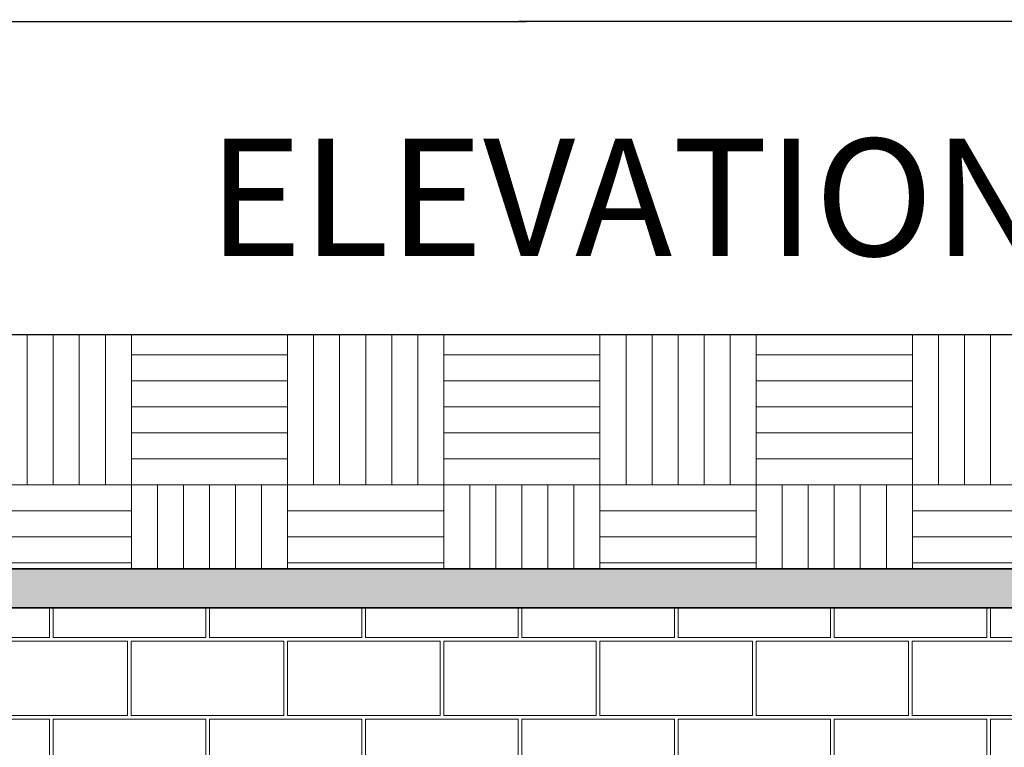
# Model space of a CAD drawing. Units: inches. Extents: x -301 to 715, y -607 to 364.
# Tile 138 of 141: x 345 to 497, y -391 to -279. Entities that reach past the tile are written whole.
import ezdxf

# ---------------------------------------------------------------- set-up
doc = ezdxf.new("R2010")
doc.units = ezdxf.units.IN
doc.header["$MEASUREMENT"] = 0
for name, color, linetype, lineweight in [('A-ANNO-DIMS', 2, 'Continuous', 18), ('A-ANNO-TITL', 1, 'Continuous', 35), ('A-ELEV', 220, 'Continuous', 30), ('A-ELEV-PATT', 4, 'Continuous', 13)]:
    doc.layers.add(name, color=color, linetype=linetype, lineweight=lineweight)
doc.styles.get("Standard").update_dxf_attribs({"font": 'arial.ttf'})
doc.dimstyles.get("Standard").update_dxf_attribs({"dimtxt": 0.18, "dimasz": 0.18, "dimexe": 0.18, "dimexo": 0.0625, "dimgap": 0.09, "dimtad": 0, "dimtih": 1, "dimtoh": 1, "dimdec": 1, "dimzin": 0, "dimdsep": 46, "dimlunit": 4, "dimtxsty": 'Standard', "dimcen": 0.09, "dimclrd": 3, "dimclre": 4, "dimclrt": 6, "dimadec": 0, "dimazin": 0, "dimtfac": 1, "dimtdec": 1, "dimtofl": 0, "dimtmove": 0, "dimatfit": 3, "dimfxl": 1, "dimtfill": 2, "dimtfillclr": 51, "dimtolj": 1, "dimtzin": 0, "dimarcsym": 0})

# ---------------------------------------------------------------- blocks, each defined once
blk = doc.blocks.new('*D192')
at = {"layer": 'A-ANNO-DIMS', "color": 4, "lineweight": -2, "transparency": 16777216}
for p, q in [((254.02, -327.49), (254.02, -279.27)), ((591.52, -327.49), (591.52, -279.27))]:
    blk.add_line(p, q, dxfattribs=at)
at = {"layer": 'A-ANNO-DIMS', "color": 3, "lineweight": -2, "transparency": 16777216}
for p, q in [((254.2, -279.45), (422.16, -279.45)), ((591.34, -279.45), (423.38, -279.45))]:
    blk.add_line(p, q, dxfattribs=at)
at = {"layer": 'A-ANNO-DIMS', "color": 3, "transparency": 16777216}
for points in [[(254.2, -279.42), (254.2, -279.48), (254.02, -279.45)], [(591.34, -279.42), (591.34, -279.48), (591.52, -279.45)]]:
    blk.add_solid(points, dxfattribs=at)
at = {"layer": 'Defpoints', "color": 0, "transparency": 16777216}
for p in [(591.52, -279.45), (254.02, -327.55), (591.52, -327.55)]:
    blk.add_point(p, dxfattribs=at)
at = {"layer": 'A-ANNO-DIMS', "color": 6, "transparency": 16777216, "insert": (422.77, -279.45), "char_height": 0.18, "attachment_point": 5, "bg_fill": 1, "box_fill_scale": 1.25, "bg_fill_color": 51, "bg_fill_transparency": 0}
blk.add_mtext('\\A1;28\'-1 1/2"', dxfattribs=at)

msp = doc.modelspace()

# ---------------------------------------------------------------- hatches: boundary and pattern name
at = {"layer": 'A-ELEV-PATT'}
h = msp.add_hatch(dxfattribs=at)
h.set_pattern_fill('AR-PARQ1', color=256, scale=2)
h.set_pattern_definition([(90, (458.62, 9.325), (-24, 24), [24, -24]), (90, (462.62, 9.325), (-24, 24), [24, -24]), (90, (466.62, 9.325), (-24, 24), [24, -24]), (90, (470.62, 9.325), (-24, 24), [24, -24]), (90, (474.62, 9.325), (-24, 24), [24, -24]), (90, (478.62, 9.325), (-24, 24), [24, -24]), (90, (482.62, 9.325), (-24, 24), [24, -24]), (0, (458.62, 33.325), (24, -24), [24, -24]), (0, (458.62, 37.325), (24, -24), [24, -24]), (0, (458.62, 41.325), (24, -24), [24, -24]), (0, (458.62, 45.325), (24, -24), [24, -24]), (0, (458.62, 49.325), (24, -24), [24, -24]), (0, (458.62, 53.325), (24, -24), [24, -24]), (0, (458.62, 57.325), (24, -24), [24, -24])])
h.paths.add_polyline_path([(264.02, -327.55), (264.02, -363.55), (581.52, -363.55), (581.52, -327.55)])
h = msp.add_hatch(color=256, dxfattribs=at)
h.dxf.hatch_style = 1
h.paths.add_polyline_path([(591.52, -363.55), (254.02, -363.55), (254.02, -369.55), (591.52, -369.55)])
h.paths.add_polyline_path([(461.02, -393.55), (413.02, -393.55), (413.02, -489.55), (461.02, -489.55)])
h.paths.add_polyline_path([(456.02, -398.55), (456.02, -484.55), (418.02, -484.55), (418.02, -398.55)], flags=16)
h.paths.add_polyline_path([(546.77, -393.55), (496.77, -393.55), (496.77, -441.55), (546.77, -441.55)])
h.paths.add_polyline_path([(501.77, -398.55), (541.77, -398.55), (541.77, -436.55), (501.77, -436.55)], flags=16)
h.paths.add_polyline_path([(360.02, -393.55), (310.02, -393.55), (310.02, -441.55), (360.02, -441.55)])
h.paths.add_polyline_path([(355.02, -398.55), (355.02, -436.55), (315.02, -436.55), (315.02, -398.55)], flags=16)
h = msp.add_hatch(dxfattribs=at)
h.set_pattern_fill('AR-B816C', color=256, scale=1.5)
h.set_pattern_definition([(0, (458.621, 9.325), (12, 12), [23.4375, -0.5625]), (0, (446.621, 9.887), (12, 12), [23.4375, -0.5625]), (90, (458.621, 9.325), (-12, 12), [-12.5625, 11.4375]), (90, (458.059, 9.325), (-12, 12), [-12.5625, 11.4375])])
h.paths.add_polyline_path([(254.02, -489.55), (413.02, -489.55), (413.02, -393.55), (461.02, -393.55), (461.02, -489.55), (591.52, -489.55), (591.52, -369.55), (254.02, -369.55)])
h.paths.add_polyline_path([(310.02, -393.55), (360.02, -393.55), (360.02, -441.55), (310.02, -441.55)], flags=16)
h.paths.add_polyline_path([(315.02, -398.55), (355.02, -398.55), (355.02, -436.55), (315.02, -436.55)], flags=0)
h.paths.add_polyline_path([(496.77, -393.55), (546.77, -393.55), (546.77, -441.55), (496.77, -441.55)], flags=16)
h.paths.add_polyline_path([(501.77, -398.55), (541.77, -398.55), (541.77, -436.55), (501.77, -436.55)], flags=0)

# ---------------------------------------------------------------- linework, layer by layer
at = {"layer": 'A-ELEV'}
for p, q in [((254.02, -327.55), (591.52, -327.55)), ((254.02, -363.55), (591.52, -363.55)), ((254.02, -369.55), (591.52, -369.55))]:
    msp.add_line(p, q, dxfattribs=at)
for points in [[(254.02, -327.55), (591.52, -327.55), (591.52, -363.55), (254.02, -363.55)], [(254.02, -363.55), (591.52, -363.55), (591.52, -369.55), (254.02, -369.55)], [(254.02, -369.55), (591.52, -369.55), (591.52, -489.55), (254.02, -489.55)]]:
    msp.add_lwpolyline(points, close=True, dxfattribs=at)

# ---------------------------------------------------------------- texts
at = {"layer": 'A-ANNO-TITL'}
msp.add_text('ELEVATION', height=18, dxfattribs=at).set_placement((374.43, -315.47))

# ---------------------------------------------------------------- dimensions: what is measured, and where the dimension line sits
at = {"layer": 'A-ANNO-DIMS'}
dim = msp.add_linear_dim(base=(591.52, -279.45), p1=(254.02, -327.55), p2=(591.52, -327.55), dimstyle='Standard', override={"dimdec": 1, "dimlfac": 1, "dimrnd": 0, "dimzin": 1, "dimdsep": 46, "dimlunit": 4, "dimfrac": 2}, dxfattribs=at)
dim.commit()
dim.dimension.update_dxf_attribs({"geometry": '*D192', "text_midpoint": (422.77, -279.45)})

doc.saveas('drawing.dxf')
